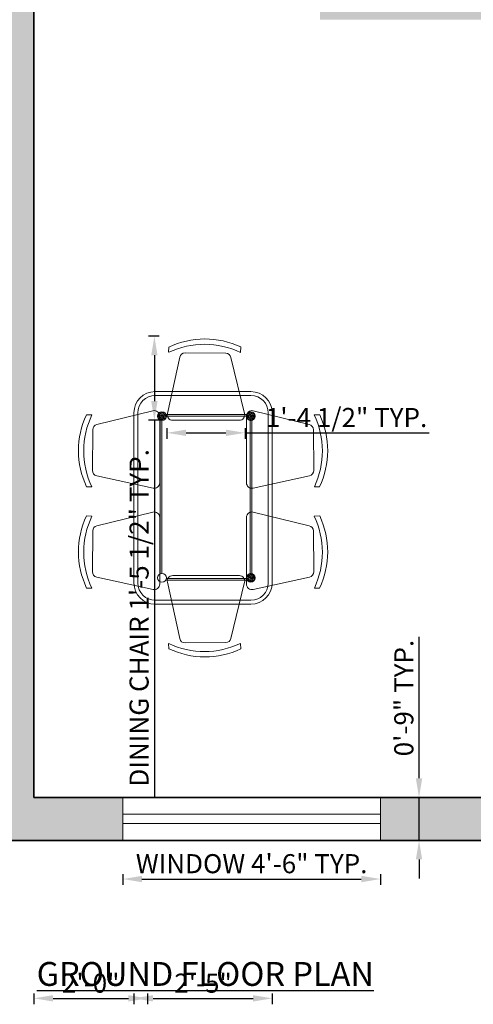
# Model space of a CAD drawing. Units: inches. Extents: x -91 to 518, y -600 to 105.
# Tile 2 of 4: x 248 to 343, y -598 to -391. Entities that reach past the tile are written whole.
import ezdxf

# ---------------------------------------------------------------- set-up
doc = ezdxf.new("R2010")
doc.units = ezdxf.units.IN
for name, color, linetype, lineweight in [('A-ANNO-DIMS', 2, 'Continuous', 18), ('A-ANNO-TITL', 7, 'Continuous', 25), ('A-FURN', 8, 'Continuous', 18), ('A-FURN-PATT', 8, 'Continuous', 13), ('A-GLAZ', 6, 'Continuous', 18), ('A-WALL', 7, 'Continuous', 35), ('A-WALL-PATT', 251, 'Continuous', 13)]:
    doc.layers.add(name, color=color, linetype=linetype, lineweight=lineweight)
doc.styles.get("Standard").update_dxf_attribs({"font": 'arial.ttf'})
doc.dimstyles.new('ISO-25', dxfattribs={"dimtxt": 4, "dimasz": 4, "dimexe": 1.25, "dimexo": 0.625, "dimtad": 1, "dimlunit": 3, "dimtxsty": 'Standard', "dimcen": 2.5, "dimadec": 0, "dimazin": 0, "dimtfac": 1, "dimtmove": 0, "dimatfit": 3, "dimfxl": 1, "dimfxlon": 1, "dimarcsym": 0})
pattern_1 = [(49.99999999999996, (324.4028617358597, -487.8748718110997), (0.2332720185709099, -0.0204086572099211), [0.0243919874784917, -0.2683118622634085]), (354.9999999999999, (324.4028617358597, -487.8748718110997), (-0.0451256105614975, 0.2446328147550751), [0.0195135899827934, -0.2146494898107268]), (100.4513999999999, (324.4223010704568, -487.876572530724), (0.1881465812661118, 0.2242240090283709), [0.0207299988847557, -0.2280299948872953]), (46.18419999999997, (324.4028617358597, -487.809826510797), (0.3470950705947874, -0.0538311696662094), [0.0365879812177375, -0.4024677933951127]), (96.6355999999998, (324.4317863204835, -487.8143124598932), (0.3039770801380951, 0.3168089454610473), [0.031094999302813, -0.3420449376928907]), (351.1842, (324.4028617358597, -487.809826510797), (0.3039768328309615, 0.3168091828844846), [0.0292703849741899, -0.3219742347160884]), (20.99999999999998, (324.4353843824411, -487.8260878361277), (0.1941299912146253, -0.1309423325295088), [0.0243919874784917, -0.2683118622634085]), (326, (324.4353843824411, -487.8260878361277), (0.079132593727417, 0.2358380109174735), [0.0195135899827934, -0.2146494898107268]), (71.45139999999996, (324.4515618832791, -487.8369997074799), (0.273262664473401, 0.1048954644957448), [0.0207299988847558, -0.2280299948872961]), (37.49999999999999, (324.4028617358597, -487.8748718110997), (0.0039547071818617, 0.1082659028576025), [0, -0.212047677813021, 0, -0.2179017548078591, 0, -0.2154625560600099]), (7.499999999999859, (324.4028617358597, -487.8748718110997), (0.0855571848434865, 0.1282731405013999), [0, -0.1242365228904509, 0, -0.2071692803173226, 0, -0.0821196911775886]), (327.5, (324.3303362241097, -487.8748718110997), (0.1736132023847377, -0.0073354419856531), [0, -0.0813066249283055, 0, -0.2536766697763131, 0, -0.3366094272031849]), (317.5, (324.2978135775284, -487.8748718110997), (0.1896675965363869, 0.0325567930077936), [0, -0.1056986124067973, 0, -0.1684673268514492, 0, -0.2390414772892185])]

# ---------------------------------------------------------------- blocks, each defined once
blk = doc.blocks.new('WIN-54IN')
for p, q in [((-8.22649996337e-05, 5.500051768139757), (53.99991773500037, 5.500051768139757)), ((-8.22649996337e-05, 3.500051768139757), (53.99991773500037, 3.500051768139757))]:
    blk.add_line(p, q)
blk.add_lwpolyline([(-8.22649996337e-05, 9.000051768139757), (53.99991773500037, 9.000051768139757), (53.99991773500037, 5.17681397576e-05), (-8.22649996337e-05, 5.17681397576e-05)], close=True)
blk = doc.blocks.new('CHAIR-DINING')
blk.add_lwpolyline([(2.792930182611542, 0.2852578078295096), (1.706859646201053, 0.3255029808819358, -0.223510425787091), (1.666634807590241, 15.41744293469554), (2.833155021222125, 15.37719776164311, 0.2259634158616322), (2.792930182611542, 0.3255029808819358, -0.2245593926962235)], format="xyb")
blk.add_lwpolyline([(2.987112122195355, 12.2711844598353), (2.920826901361976, 3.749227795311924, 0.354444779783923), (3.820568093279405, 2.62163963949348), (15.64168084863621, 0.0270928925841076, 0.4790082601800635), (17.03252172073934, 1.145772916677572), (17.03252172073934, 15.12664748537537, 0.4860847710136459), (15.61606314851491, 16.2393957816692), (3.861235597671964, 13.37502462389415, 0.3436426597751999)], format="xyb", close=True)
blk = doc.blocks.new('*D16')
at = {"layer": 'A-ANNO-DIMS', "color": 0, "lineweight": -2, "transparency": 16777216}
for p, q in [((269.1846508389144, -570.3577049396689), (269.1846508389144, -572.6077049396689)), ((273.1846508389144, -571.3577049396689), (319.1846508389144, -571.3577049396689)), ((323.1846508389144, -570.3577049396689), (323.1846508389144, -572.6077049396689))]:
    blk.add_line(p, q, dxfattribs=at)
at = {"layer": 'A-ANNO-DIMS', "color": 0, "transparency": 16777216}
for points in [[(273.1846508389144, -570.6910382730022), (273.1846508389144, -572.0243716063355), (269.1846508389144, -571.3577049396689)], [(319.1846508389144, -570.6910382730022), (319.1846508389144, -572.0243716063355), (323.1846508389144, -571.3577049396689)]]:
    blk.add_solid(points, dxfattribs=at)
at = {"layer": 'Defpoints', "color": 0, "transparency": 16777216}
for p in [(269.1846508389144, -563.2577049396688), (323.1846508389144, -563.2577049396688), (323.1846508389144, -571.3577049396689)]:
    blk.add_point(p, dxfattribs=at)
at = {"layer": 'A-ANNO-DIMS', "color": 0, "transparency": 16777216, "insert": (296.1846508389144, -568.6631278591777), "char_height": 4, "attachment_point": 5}
blk.add_mtext('WINDOW 4\'-6" TYP.', dxfattribs=at)
blk = doc.blocks.new('*D17')
at = {"layer": 'A-ANNO-DIMS', "color": 0, "lineweight": -2, "transparency": 16777216}
for p, q in [((331.2846508389147, -550.257704939669), (331.2846508389147, -520.625713125208)), ((330.2846508389147, -554.257704939669), (332.5346508389147, -554.257704939669)), ((331.2846508389147, -563.2577049396691), (331.2846508389147, -554.257704939669)), ((330.2846508389147, -563.2577049396691), (332.5346508389147, -563.2577049396691)), ((331.2846508389147, -567.2577049396691), (331.2846508389147, -571.2577049396691))]:
    blk.add_line(p, q, dxfattribs=at)
at = {"layer": 'A-ANNO-DIMS', "color": 0, "transparency": 16777216}
for points in [[(330.617984172248, -550.257704939669), (331.9513175055814, -550.257704939669), (331.2846508389147, -554.257704939669)], [(330.617984172248, -567.2577049396691), (331.9513175055814, -567.2577049396691), (331.2846508389147, -563.2577049396691)]]:
    blk.add_solid(points, dxfattribs=at)
at = {"layer": 'Defpoints', "color": 0, "transparency": 16777216}
for p in [(323.1846508389145, -554.257704939669), (331.2846508389147, -554.257704939669), (323.1846508389145, -563.2577049396691)]:
    blk.add_point(p, dxfattribs=at)
at = {"layer": 'A-ANNO-DIMS', "color": 0, "transparency": 16777216, "insert": (328.6173588880277, -533.4417090324386), "char_height": 4, "attachment_point": 5, "rotation": 90}
blk.add_mtext('0\'-9" TYP.', dxfattribs=at)
blk = doc.blocks.new('*D24')
at = {"layer": 'A-ANNO-DIMS', "color": 0, "lineweight": -2, "transparency": 16777216}
for p, q in [((276.7933076695092, -457.6302889957347), (274.5433076695092, -457.6302889957347)), ((275.7933076695092, -461.6302889957347), (275.7933076695092, -471.2322414157476)), ((276.7933076695092, -475.2322414157476), (274.5433076695092, -475.2322414157476)), ((275.7933076695092, -475.2322414157476), (275.7933076695092, -554.0347652902359))]:
    blk.add_line(p, q, dxfattribs=at)
at = {"layer": 'A-ANNO-DIMS', "color": 0, "transparency": 16777216}
for points in [[(275.1266410028425, -461.6302889957347), (276.4599743361759, -461.6302889957347), (275.7933076695092, -457.6302889957347)], [(275.1266410028425, -471.2322414157476), (276.4599743361759, -471.2322414157476), (275.7933076695092, -475.2322414157476)]]:
    blk.add_solid(points, dxfattribs=at)
at = {"layer": 'Defpoints', "color": 0, "transparency": 16777216}
for p in [(278.4336005333661, -457.6302889957347), (275.7933076695092, -475.2322414157476), (278.4336005316559, -475.2322414157476)]:
    blk.add_point(p, dxfattribs=at)
at = {"layer": 'A-ANNO-DIMS', "color": 0, "transparency": 16777216, "insert": (273.1000948454981, -516.6335033529917), "char_height": 4, "attachment_point": 5, "rotation": 90}
blk.add_mtext('DINING CHAIR 1\'-5 1/2" TYP.', dxfattribs=at)
blk = doc.blocks.new('*D25')
at = {"layer": 'A-ANNO-DIMS', "color": 0, "lineweight": -2, "transparency": 16777216}
for p, q in [((278.4336005316558, -476.8725342795447), (278.4336005316558, -479.1225342795446)), ((282.4336005316558, -477.8725342795446), (290.8034790113715, -477.8725342795446)), ((294.8034790113716, -476.8725342795447), (294.8034790113716, -479.1225342795446)), ((294.8034790113716, -477.8725342795446), (333.3795363101438, -477.8725342795446))]:
    blk.add_line(p, q, dxfattribs=at)
at = {"layer": 'A-ANNO-DIMS', "color": 0, "transparency": 16777216}
for points in [[(282.4336005316558, -477.2058676128779), (282.4336005316558, -478.5392009462113), (278.4336005316558, -477.8725342795446)], [(290.8034790113715, -477.2058676128779), (290.8034790113715, -478.5392009462113), (294.8034790113716, -477.8725342795446)]]:
    blk.add_solid(points, dxfattribs=at)
at = {"layer": 'Defpoints', "color": 0, "transparency": 16777216}
for p in [(278.4336005316558, -475.2322414157474), (294.8034790113716, -475.2322414173379), (294.8034790113716, -477.8725342795446)]:
    blk.add_point(p, dxfattribs=at)
at = {"layer": 'A-ANNO-DIMS', "color": 0, "transparency": 16777216, "insert": (316.0915076607576, -475.1793214555337), "char_height": 4, "attachment_point": 5}
blk.add_mtext('1\'-4 1/2" TYP.', dxfattribs=at)
blk = doc.blocks.new('*D35')
at = {"layer": 'A-ANNO-DIMS', "color": 0, "lineweight": -2, "transparency": 16777216}
for p, q in [((-81.98865400000005, -381.3071320000002), (-81.98865400000005, -377.3071320000003)), ((-80.98865400000004, -385.3071320000003), (-83.23865400000004, -385.3071320000003)), ((-81.98865400000005, -385.3071320000003), (-81.98865400000005, -391.3071320000003)), ((-80.98865400000004, -391.3071320000003), (-83.23865400000004, -391.3071320000003)), ((-81.98865400000005, -395.3071320000003), (-81.98865400000005, -411.1901470068215))]:
    blk.add_line(p, q, dxfattribs=at)
at = {"layer": 'A-ANNO-DIMS', "color": 0, "transparency": 16777216}
for points in [[(-82.65532066666673, -381.3071320000002), (-81.32198733333337, -381.3071320000002), (-81.98865400000005, -385.3071320000003)], [(-82.65532066666673, -395.3071320000003), (-81.32198733333337, -395.3071320000003), (-81.98865400000005, -391.3071320000003)]]:
    blk.add_solid(points, dxfattribs=at)
at = {"layer": 'Defpoints', "color": 0, "transparency": 16777216}
for p in [(310.5439730000001, -385.3071320000002), (-81.98865400000005, -391.3071320000003), (310.5439730000001, -391.3071320000002)]:
    blk.add_point(p, dxfattribs=at)
at = {"layer": 'A-ANNO-DIMS', "color": 0, "transparency": 16777216, "insert": (-84.65594595088692, -405.2486395034108), "char_height": 4, "attachment_point": 5, "rotation": 90}
blk.add_mtext('0\'-6"', dxfattribs=at)
blk = doc.blocks.new('*D37')
at = {"layer": 'A-ANNO-DIMS', "color": 0, "lineweight": -2, "transparency": 16777216}
for p, q in [((-80.98865400000005, -530.3071320000003), (-83.23865400000007, -530.3071320000003)), ((-81.98865400000005, -534.3071320000003), (-81.98865400000004, -550.3071320000003)), ((-80.98865400000005, -554.3071320000003), (-83.23865400000005, -554.3071320000003))]:
    blk.add_line(p, q, dxfattribs=at)
at = {"layer": 'A-ANNO-DIMS', "color": 0, "transparency": 16777216}
for points in [[(-82.65532066666673, -534.3071320000003), (-81.32198733333337, -534.3071320000003), (-81.98865400000005, -530.3071320000003)], [(-82.6553206666667, -550.3071320000003), (-81.32198733333337, -550.3071320000003), (-81.98865400000004, -554.3071320000003)]]:
    blk.add_solid(points, dxfattribs=at)
at = {"layer": 'Defpoints', "color": 0, "transparency": 16777216}
for p in [(375.0870760000001, -530.3071320000003), (-81.98865400000004, -554.3071320000003), (375.0870760000001, -554.3071320000003)]:
    blk.add_point(p, dxfattribs=at)
at = {"layer": 'A-ANNO-DIMS', "color": 0, "transparency": 16777216, "insert": (-84.65594595088695, -542.3071320000003), "char_height": 4, "attachment_point": 5, "rotation": 90}
blk.add_mtext('2\'-0"', dxfattribs=at)
blk = doc.blocks.new('*D46')
at = {"layer": 'A-ANNO-DIMS', "color": 0, "lineweight": -2, "transparency": 16777216}
for p, q in [((250.5439729999999, -595.357132), (250.5439729999999, -597.6071319999999)), ((274.3406869999999, -595.357132), (274.3406869999999, -597.6071319999999)), ((254.543973, -596.3571319999999), (270.3406869999999, -596.3571319999999))]:
    blk.add_line(p, q, dxfattribs=at)
at = {"layer": 'A-ANNO-DIMS', "color": 0, "transparency": 16777216}
for points in [[(254.543973, -595.6904653333333), (254.543973, -597.0237986666666), (250.5439729999999, -596.3571319999999)], [(270.3406869999999, -595.6904653333333), (270.3406869999999, -597.0237986666666), (274.3406869999999, -596.3571319999999)]]:
    blk.add_solid(points, dxfattribs=at)
at = {"layer": 'Defpoints', "color": 0, "transparency": 16777216}
for p in [(250.543973, 3.692867999999999), (274.340687, 3.692867999999999), (274.3406869999999, -596.3571319999999)]:
    blk.add_point(p, dxfattribs=at)
at = {"layer": 'A-ANNO-DIMS', "color": 0, "transparency": 16777216, "insert": (262.44233, -593.6898400491132), "char_height": 4, "attachment_point": 5}
blk.add_mtext('2\'-0"', dxfattribs=at)
blk = doc.blocks.new('*D50')
at = {"layer": 'A-ANNO-DIMS', "color": 0, "lineweight": -2, "transparency": 16777216}
for p, q in [((-80.9886540000001, -391.3071320000003), (-83.2386540000001, -391.3071320000003)), ((-81.98865400000007, -395.3071320000003), (-81.98865400000005, -452.1362110000002)), ((-80.98865400000008, -456.1362110000002), (-83.23865400000007, -456.1362110000002))]:
    blk.add_line(p, q, dxfattribs=at)
at = {"layer": 'A-ANNO-DIMS', "color": 0, "transparency": 16777216}
for points in [[(-82.65532066666674, -395.3071320000003), (-81.3219873333334, -395.3071320000003), (-81.98865400000007, -391.3071320000003)], [(-82.65532066666673, -452.1362110000002), (-81.32198733333337, -452.1362110000002), (-81.98865400000005, -456.1362110000002)]]:
    blk.add_solid(points, dxfattribs=at)
at = {"layer": 'Defpoints', "color": 0, "transparency": 16777216}
for p in [(472.5439730000002, -391.3071320000002), (-81.98865400000005, -456.1362110000002), (472.5439730000002, -456.1362110000002)]:
    blk.add_point(p, dxfattribs=at)
at = {"layer": 'A-ANNO-DIMS', "color": 0, "transparency": 16777216, "insert": (-84.64776041200562, -423.7216715000001), "char_height": 4, "attachment_point": 5, "rotation": 90}
blk.add_mtext('5\'-5"', dxfattribs=at)
blk = doc.blocks.new('*D51')
at = {"layer": 'A-ANNO-DIMS', "color": 0, "lineweight": -2, "transparency": 16777216}
for p, q in [((250.543973, 95.58768199999997), (250.543973, 97.83768199999997)), ((269.184651, 95.58768199999997), (269.184651, 97.83768199999997)), ((254.543973, 96.587682), (265.184651, 96.587682)), ((269.184651, 96.587682), (294.0117314911324, 96.587682))]:
    blk.add_line(p, q, dxfattribs=at)
at = {"layer": 'A-ANNO-DIMS', "color": 0, "transparency": 16777216}
for points in [[(254.543973, 97.25434866666667), (254.543973, 95.92101533333332), (250.543973, 96.587682)], [(265.184651, 97.25434866666667), (265.184651, 95.92101533333332), (269.184651, 96.587682)]]:
    blk.add_solid(points, dxfattribs=at)
at = {"layer": 'Defpoints', "color": 0, "transparency": 16777216}
for p in [(269.184651, 96.587682), (250.543973, -554.307132), (269.184651, -554.257705)]:
    blk.add_point(p, dxfattribs=at)
at = {"layer": 'A-ANNO-DIMS', "color": 0, "transparency": 16777216, "insert": (283.5981912455661, 99.28089482401091), "char_height": 4, "attachment_point": 5}
blk.add_mtext('1\'-6 1/2"', dxfattribs=at)
blk = doc.blocks.new('*D54')
at = {"layer": 'A-ANNO-DIMS', "color": 0, "lineweight": -2, "transparency": 16777216}
for p, q in [((271.510191, -595.357132), (271.510191, -597.6071319999999)), ((300.491835, -595.357132), (300.491835, -597.6071319999999)), ((275.510191, -596.3571319999999), (296.491835, -596.3571319999999))]:
    blk.add_line(p, q, dxfattribs=at)
at = {"layer": 'A-ANNO-DIMS', "color": 0, "transparency": 16777216}
for points in [[(275.510191, -595.6904653333333), (275.510191, -597.0237986666666), (271.510191, -596.3571319999999)], [(296.491835, -595.6904653333333), (296.491835, -597.0237986666666), (300.491835, -596.3571319999999)]]:
    blk.add_solid(points, dxfattribs=at)
at = {"layer": 'Defpoints', "color": 0, "transparency": 16777216}
for p in [(271.510191, -509.320483), (300.491835, -509.320483), (300.491835, -596.3571319999999)]:
    blk.add_point(p, dxfattribs=at)
at = {"layer": 'A-ANNO-DIMS', "color": 0, "transparency": 16777216, "insert": (286.001013, -593.6898400491132), "char_height": 4, "attachment_point": 5}
blk.add_mtext('2\'-5"', dxfattribs=at)
blk = doc.blocks.new('*D55')
at = {"layer": 'A-ANNO-DIMS', "color": 0, "lineweight": -2, "transparency": 16777216}
for p, q in [((513.5939730000003, -469.2346910000002), (515.8439730000003, -469.2346910000002)), ((514.5939730000003, -473.2346910000002), (514.5939730000003, -509.7744600000002)), ((513.5939730000003, -513.7744600000002), (515.8439730000003, -513.7744600000002))]:
    blk.add_line(p, q, dxfattribs=at)
at = {"layer": 'A-ANNO-DIMS', "color": 0, "transparency": 16777216}
for points in [[(513.9273063333338, -473.2346910000002), (515.260639666667, -473.2346910000002), (514.5939730000003, -469.2346910000002)], [(513.9273063333338, -509.7744600000002), (515.260639666667, -509.7744600000002), (514.5939730000003, -513.7744600000002)]]:
    blk.add_solid(points, dxfattribs=at)
at = {"layer": 'Defpoints', "color": 0, "transparency": 16777216}
for p in [(296.0378580000001, -469.2346910000002), (296.0378580000001, -513.7744600000002), (514.5939730000003, -513.7744600000002)]:
    blk.add_point(p, dxfattribs=at)
at = {"layer": 'A-ANNO-DIMS', "color": 0, "transparency": 16777216, "insert": (511.8993959195091, -491.5045755000003), "char_height": 4, "attachment_point": 5, "rotation": 90}
blk.add_mtext('3\'-8 1/2"', dxfattribs=at)

msp = doc.modelspace()

# ---------------------------------------------------------------- hatches: boundary and pattern name
at = {"layer": 'A-FURN-PATT'}
h = msp.add_hatch(dxfattribs=at)
h.set_pattern_fill('AR-CONC,_I', color=256, scale=0.0325226499713223, angle=-1.27e-14, style=2)
h.set_pattern_definition(pattern_1)
edge = h.paths.add_edge_path()
edge.add_arc((277.3838618285608, -474.3810002883932), 0.9317545682717732, 0, 360)
h = msp.add_hatch(dxfattribs=at)
h.set_pattern_fill('AR-CONC,_I', color=256, scale=0.0325226499713223, angle=-1.27e-14, style=2)
h.set_pattern_definition(pattern_1)
edge = h.paths.add_edge_path()
edge.add_arc((296.0189697946682, -474.3810002883932), 0.9317545682717732, 0, 360)
h = msp.add_hatch(dxfattribs=at)
h.set_pattern_fill('AR-CONC,_I', color=256, scale=0.0325226499713223, angle=-1.27e-14, style=2)
h.set_pattern_definition(pattern_1)
edge = h.paths.add_edge_path()
edge.add_arc((277.3838618285608, -508.2535558770147), 0.9317545682717732, -1.27e-14, 360)
h.paths.add_polyline_path([(275.8405406483935, -507.1060460311206), (275.8994321209761, -507.1060460311206), (275.8994321209761, -507.0837761465219), (275.8405406483935, -507.0837761465219)], flags=9)
h = msp.add_hatch(dxfattribs=at)
h.set_pattern_fill('AR-CONC,_I', color=256, scale=0.0325226499713223, angle=-1.27e-14, style=2)
h.set_pattern_definition(pattern_1)
edge = h.paths.add_edge_path()
edge.add_arc((296.0189697946682, -508.2535558770147), 0.9317545682717732, 0, 360)
at = {"layer": 'A-WALL-PATT'}
h = msp.add_hatch(color=256, dxfattribs=at)
h.dxf.hatch_style = 1
h.paths.add_polyline_path([(10.54397302627791, 3.69286819609001), (34.46210501665792, 3.692868196090003), (34.46210501665792, 12.69286819609001), (1.54397302627791, 12.69286819609001), (1.54397302627791, -180.8777568066362), (10.54397302627791, -180.8777568066362)])
h.paths.add_polyline_path([(46.54397302627785, -92.30713180391), (10.54397302627791, -92.30713180390997), (10.54397302627791, -98.30713180391), (46.54397302627785, -98.30713180391001)])
h.paths.add_polyline_path([(130.3809177350003, 12.69286819608999), (52.46210501665791, 12.69286819608999), (52.46210501665792, 3.692868196090003), (82.54397302627785, 3.692868196090003), (88.54397302627785, 3.692868196090003), (130.3809177350004, 3.692868196090003)])
h.paths.add_polyline_path([(88.5439730262779, 3.692868196089996), (82.54397302627792, 3.692868196089996), (82.54397302627792, -92.30713180390997), (76.54397302627785, -92.30713180391001), (76.54397302627785, -94.37012392989423), (76.54397302627785, -98.30713180391001), (82.5439730262779, -98.30713180391), (82.5439730262779, -106.0567926816102), (85.5222416603892, -106.0567926816102), (88.54397302627791, -106.0567926816102)])
h.paths.add_polyline_path([(250.5439730262778, -146.30713180391), (245.7716552283821, -146.30713180391), (244.5439730262779, -146.30713180391), (244.5439730262779, -152.30713180391), (88.54397302627791, -152.3071318039099), (88.54397302627791, -141.7441975357105), (85.71753115439951, -141.7441975357105), (82.54397302627792, -141.7441975357105), (82.54397302627792, -152.3071318039099), (10.54397302627791, -152.3071318039099), (10.54397302627791, -158.30713180391), (88.54397302627785, -158.30713180391), (118.5439730262778, -158.30713180391), (118.5439730262778, -164.30713180391), (120.6069651522621, -164.30713180391), (124.5439730262778, -164.30713180391), (124.5439730262778, -158.3071318039099), (244.5439730262779, -158.30713180391), (244.5439730262779, -164.30713180391), (250.5439730262779, -164.30713180391)])
h.paths.add_polyline_path([(274.3406872340411, 12.69286819609), (184.3809177350003, 12.69286819609), (184.3809177350003, 3.692868196089996), (244.5439730262779, 3.692868196089996), (250.5439730262779, 3.692868196089996), (274.3406872340411, 3.692868196090003)])
h.paths.add_polyline_path([(250.5439730262779, 3.692868196090003), (244.5439730262779, 3.692868196089989), (244.5439730262779, -110.30713180391), (250.5439730262779, -110.30713180391), (250.5439730262779, -98.30713180391), (310.5439730262779, -98.30713180391001), (310.5439730262779, -110.30713180391), (316.5439730262779, -110.30713180391), (316.5439730262779, -86.51662232277216), (312.6069651522621, -86.51662232277216), (310.5439730262779, -86.51662232277216), (310.543973026278, -92.30713180391001), (250.5439730262779, -92.30713180390997)])
h.paths.add_polyline_path([(481.5439730262779, 12.69286819608999), (292.3406872340411, 12.69286819609), (292.3406872340411, 3.692868196089989), (310.5439730262779, 3.692868196089996), (316.5439730262779, 3.692868196089996), (472.5439730262779, 3.692868196089989), (472.5439730262778, -34.12947996685534), (481.5439730262779, -34.12947996685534)])
h.paths.add_polyline_path([(316.5439730262779, 3.692868196090003), (310.5439730262779, 3.692868196089996), (310.5439730262779, -56.51662232277216), (316.5439730262779, -56.51662232277216)], flags=17)
h.paths.add_polyline_path([(481.543973026278, -88.12947996685536), (472.5439730262779, -88.12947996685536), (472.5439730262779, -189.4514204144393), (481.5439730262779, -189.4514204144393)])
h.paths.add_polyline_path([(472.5439730262779, -152.30713180391), (316.5439730262779, -152.30713180391), (316.5439730262779, -146.30713180391), (315.3190113957458, -146.30713180391), (310.5439730262779, -146.30713180391), (310.5439730262779, -260.30713180391), (316.543973026278, -260.30713180391), (316.5439730262779, -158.30713180391), (472.5439730262778, -158.30713180391)])
h.paths.add_polyline_path([(481.5439730262779, -243.4514204144393), (472.5439730262778, -243.4514204144393), (472.5439730262779, -308.30713180391), (472.5439730262779, -332.5934456982646), (481.5439730262779, -332.5934456982646)])
h.paths.add_polyline_path([(472.543973026278, -302.30713180391), (316.5439730262779, -302.30713180391), (316.543973026278, -296.30713180391), (315.3223312342462, -296.30713180391), (310.5439730262779, -296.30713180391), (310.5439730262779, -308.3071318039099), (472.543973026278, -308.3071318039101)])
h.paths.add_polyline_path([(481.543973026278, -366.5934456982646), (472.5439730262779, -366.5934456982645), (472.5439730262779, -385.30713180391), (472.5439730262779, -456.1362109337742), (481.5439730262779, -456.1362109337742)])
h.paths.add_polyline_path([(472.543973026278, -385.3071318039099), (310.543973026278, -385.30713180391), (310.5439730262779, -391.30713180391), (472.543973026278, -391.30713180391)])
h.paths.add_polyline_path([(481.543973026278, -510.1362109337741), (472.5439730262779, -510.1362109337741), (472.5439730262778, -554.30713180391), (323.1846508389144, -554.30713180391), (323.1846508389144, -563.30713180391), (481.5439730262779, -563.30713180391)])
h.paths.add_polyline_path([(250.5439730262778, -384.7238270396974), (229.6450614403802, -384.7238270396974), (229.6450614403802, -393.7238270396975), (241.5439730262779, -393.7238270396974), (241.5439730262779, -563.30713180391), (269.1846508389144, -563.30713180391), (269.1846508389144, -554.30713180391), (250.5439730262779, -554.30713180391)])
h.paths.add_polyline_path([(195.6450614403802, -384.7238270396974), (133.7004703433376, -384.7238270396974), (133.7004703433376, -393.7238270396974), (195.6450614403802, -393.7238270396975)])
h.paths.add_polyline_path([(99.70047034333766, -384.7238270396975), (61.54397302627785, -384.7238270396975), (61.54397302627785, -391.562077029412), (61.33486888165797, -393.7238270396973), (77.04231968784188, -393.7238270396973), (99.70047034333767, -393.7238270396973)])
h.paths.add_polyline_path([(10.54397302627791, -264.0141460456657), (1.54397302627791, -264.0141460456657), (1.543973026277911, -330.0475231407777), (10.54397302627791, -330.0475231407777)])
h.paths.add_polyline_path([(10.54397302627791, -198.8777568066362), (1.54397302627791, -198.8777568066361), (1.543973026277911, -230.0141460456657), (10.54397302627791, -230.0141460456657)])
h.paths.add_polyline_path([(208.5439730262779, -218.30713180391), (124.5439730262779, -218.30713180391), (124.5439730262778, -194.30713180391), (118.5439730262778, -194.30713180391), (118.5439730262778, -218.30713180391), (10.54397302627791, -218.30713180391), (10.54397302627791, -224.30713180391), (118.5439730262778, -224.30713180391), (124.5439730262778, -224.30713180391), (208.5439730262778, -224.30713180391)])
h.paths.add_polyline_path([(250.5439730262778, -194.30713180391), (244.5439730262779, -194.30713180391), (244.5439730262779, -218.30713180391), (238.5439730262779, -218.30713180391), (238.5439730262779, -224.30713180391), (244.5439730262779, -224.30713180391), (244.5439730262778, -384.7238270396974), (250.5439730262779, -384.7238270396975)])

# ---------------------------------------------------------------- linework, layer by layer
at = {"layer": 'A-FURN'}
for p, q in [((275.9641683257291, -469.2346911229166), (296.0378582144049, -469.2346911229166)), ((275.9641683257291, -470.0477573721106), (296.0378582144049, -470.0477573721106)), ((271.5101914141485, -509.3204833449934), (271.5101914141485, -473.6886680365374)), ((272.3232576684422, -509.3204833449934), (272.3232576684422, -473.6886680365374)), ((295.0675219689576, -474.0518375842498), (278.3488114216488, -474.0518375842498)), ((295.0675219689576, -474.3770640837234), (278.3488114216488, -474.3770640837234)), ((299.6787688798518, -473.6886680365374), (299.6787688798518, -509.3204833449934)), ((300.4918351259858, -473.6886680365374), (300.4918351259858, -509.3204833449934)), ((277.0164369245863, -475.3835361278933), (277.0164369245863, -507.3893375609479)), ((277.34166342304, -475.3835361278933), (277.34166342304, -507.3893375609479)), ((295.8732423653853, -507.3893375609479), (295.8732423653853, -475.3835361278933)), ((296.198468863839, -507.3893375609479), (296.198468863839, -475.3835361278933)), ((278.3488114216488, -508.3958096046079), (295.0675219689576, -508.3958096046079)), ((278.3488114216488, -508.7210361045915), (295.0675219689576, -508.7210361045915)), ((296.0378582144049, -512.9613940094202), (275.9641683257291, -512.9613940094202)), ((296.0378582144049, -513.7744602586142), (275.9641683257291, -513.7744602586142))]:
    msp.add_line(p, q, dxfattribs=at)
for centre in [(277.3838618285608, -474.3810002883932), (296.0189697946682, -474.3810002883932), (277.3838618285608, -508.2535558770147), (296.0189697946682, -508.2535558770147)]:
    msp.add_circle(centre, 0.9317545682717732, dxfattribs=at)
for centre, radius, start, end in [((275.9641683257291, -473.6886680365374), 4.453976913572581, 90, 180), ((275.9641683257291, -473.6886680365374), 3.640910664289525, 90, 180), ((296.0378582144049, -473.6886680365374), 4.453976913572581, 0, 90), ((296.0378582144049, -473.6886680365374), 3.640910664289525, 0, 90), ((275.9641683257291, -509.3204833449934), 4.453976913572581, 180, 270), ((275.9641683257291, -509.3204833449934), 3.640910664289525, 180, 270), ((296.0378582144049, -509.3204833449934), 4.453976913572581, 270, 0), ((296.0378582144049, -509.3204833449934), 3.640910664289525, 270, 0)]:
    msp.add_arc(centre, radius, start, end, dxfattribs=at)
at = {"layer": 'A-WALL'}
for p, q in [((250.5439730262779, -554.30713180391), (250.5439730262779, -194.30713180391)), ((472.5439730262778, -554.30713180391), (250.5439730262779, -554.30713180391)), ((481.5439730262779, -563.30713180391), (1.54397302627791, -563.30713180391))]:
    msp.add_line(p, q, dxfattribs=at)

# ---------------------------------------------------------------- block references
at = {"layer": 'A-FURN', "rotation": 269.9999999944331}
msp.add_blockref('CHAIR-DINING', (278.4808701960909, -458.1997196948519), dxfattribs=at)
at = {"layer": 'A-FURN'}
for p in [(259.868, -489.487), (259.8680000000001, -510.7091758066415)]:
    msp.add_blockref('CHAIR-DINING', p, dxfattribs=at)
at = {"layer": 'A-FURN', "extrusion": (0, 0, -1), "zscale": -1}
for p in [(-312.1340265431005, -489.4870000000988), (-312.1340265431004, -510.7091758067405)]:
    msp.add_blockref('CHAIR-DINING', p, dxfattribs=at)
at = {"layer": 'A-FURN', "extrusion": (0, 0, -1), "zscale": -1, "rotation": 89.9999999943933}
msp.add_blockref('CHAIR-DINING', (-278.4808701960745, -524.8094316868971), dxfattribs=at)
at = {"layer": 'A-GLAZ'}
msp.add_blockref('WIN-54IN', (269.184733103914, -563.2577567078087), dxfattribs=at)

# ---------------------------------------------------------------- texts
at = {"layer": 'A-ANNO-TITL', "insert": (251.1092637156498, -588.7453900146859), "char_height": 5, "attachment_point": 1}
msp.add_mtext_dynamic_manual_height_columns('{\\LGROUND FLOOR PLAN}', width=224.7349320721896, gutter_width=12.5, heights=[0], dxfattribs=at)

# ---------------------------------------------------------------- dimensions: what is measured, and where the dimension line sits
at = {"layer": 'A-ANNO-DIMS'}
for base, p1, p2, picture, middle in [((269.184651, 96.587682), (250.543973, -554.307132), (269.184651, -554.257705), '*D51', (283.5981912455661, 99.28089482401091)), ((274.3406869999999, -596.3571319999999), (250.543973, 3.692867999999999), (274.340687, 3.692867999999999), '*D46', (262.44233, -593.6898400491132)), ((300.491835, -596.3571319999999), (271.510191, -509.320483), (300.491835, -509.320483), '*D54', (286.001013, -593.6898400491132))]:
    dim = msp.add_linear_dim(base=base, p1=p1, p2=p2, dimstyle='ISO-25', override={"dimdec": 1, "dimlfac": 1, "dimrnd": 0, "dimzin": 1, "dimdsep": 46, "dimlunit": 4, "dimfrac": 2}, dxfattribs=at)
    dim.commit()
    dim.dimension.update_dxf_attribs({"geometry": picture, "text_midpoint": middle})
for base, p1, p2, picture, middle in [((-81.98865400000005, -391.3071320000003), (310.543973, -385.307132), (310.543973, -391.307132), '*D35', (-84.65594595088692, -405.2486395034108)), ((-81.98865400000005, -456.1362110000002), (472.5439729999999, -391.307132), (472.5439729999999, -456.136211), '*D50', (-84.64776041200562, -423.7216715000001)), ((514.5939730000003, -513.7744600000002), (296.037858, -469.234691), (296.037858, -513.7744599999999), '*D55', (511.8993959195091, -491.5045755000003)), ((-81.98865400000004, -554.3071320000003), (375.087076, -530.3071319999999), (375.087076, -554.307132), '*D37', (-84.65594595088695, -542.3071320000003))]:
    dim = msp.add_linear_dim(base=base, p1=p1, p2=p2, angle=90, dimstyle='ISO-25', override={"dimdec": 1, "dimlfac": 1, "dimrnd": 0, "dimzin": 1, "dimdsep": 46, "dimlunit": 4, "dimfrac": 2}, dxfattribs=at)
    dim.commit()
    dim.dimension.update_dxf_attribs({"geometry": picture, "text_midpoint": middle})
for base, p1, p2, angle, text, picture, middle in [((275.7933076695092, -475.2322414157476), (278.433600533366, -457.6302889957346), (278.4336005316558, -475.2322414157474), 269.999999994433, 'DINING CHAIR <> TYP.', '*D24', (273.1000948454981, -516.6335033529917)), ((294.8034790113716, -477.8725342795446), (278.4336005316558, -475.2322414157474), (294.8034790113716, -475.2322414173379), 359.999999994433, '<> TYP.', '*D25', (316.0915076607576, -475.1793214555337)), ((331.2846508389147, -554.257704939669), (323.1846508389144, -563.2577049396688), (323.1846508389144, -554.2577049396689), 90, '<> TYP.', '*D17', (328.6173588880277, -533.4417090324386))]:
    dim = msp.add_linear_dim(base=base, p1=p1, p2=p2, angle=angle, text=text, dimstyle='ISO-25', override={"dimdec": 1, "dimlfac": 1, "dimrnd": 0, "dimzin": 1, "dimdsep": 46, "dimlunit": 4, "dimfrac": 2}, dxfattribs=at)
    dim.commit()
    dim.dimension.update_dxf_attribs({"geometry": picture, "text_midpoint": middle})
dim = msp.add_linear_dim(base=(323.1846508389144, -571.3577049396689), p1=(269.1846508389144, -563.2577049396688), p2=(323.1846508389144, -563.2577049396688), text='WINDOW <> TYP.', dimstyle='ISO-25', override={"dimdec": 1, "dimlfac": 1, "dimrnd": 0, "dimzin": 1, "dimdsep": 46, "dimlunit": 4, "dimfrac": 2}, dxfattribs=at)
dim.commit()
dim.dimension.update_dxf_attribs({"geometry": '*D16', "text_midpoint": (296.1846508389144, -568.6631278591777)})

doc.saveas('drawing.dxf')
